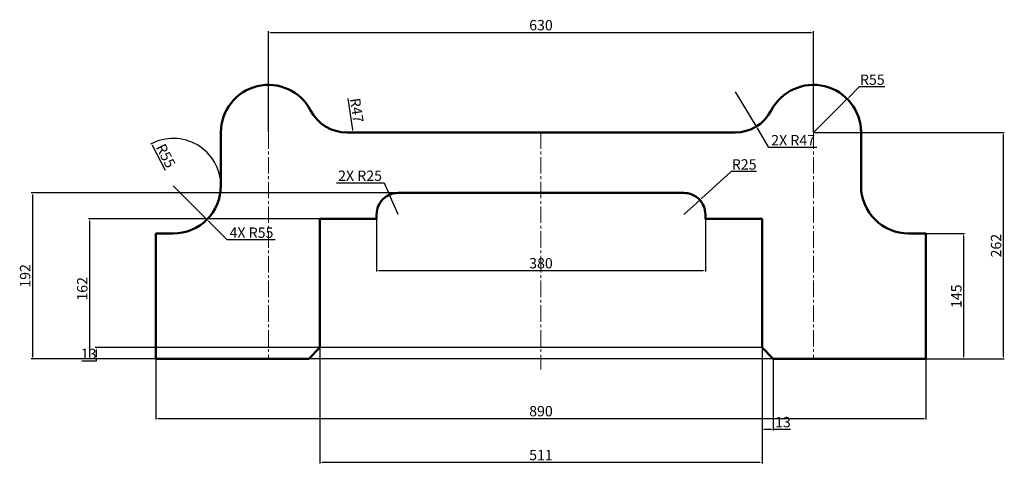
# Model space of a CAD drawing. Units: millimetres. Extents: x 47 to 1186, y 220 to 733.
import ezdxf

# ---------------------------------------------------------------- set-up
doc = ezdxf.new("R2010")
doc.units = ezdxf.units.MM
doc.linetypes.add('CENTER2', pattern=[28.575, 19.05, -3.175, 3.175, -3.175])
for name, color, linetype, lineweight in [('M-CNTR', 4, 'CENTER2', 18), ('M-DIMS', 2, 'Continuous', 25), ('M-OUTL', 7, 'Continuous', 50)]:
    doc.layers.add(name, color=color, linetype=linetype, lineweight=lineweight)
doc.styles.get("Standard").update_dxf_attribs({"font": 'arial.ttf'})
doc.dimstyles.new('ISO-25', dxfattribs={"dimtxt": 12, "dimasz": 2.5, "dimexe": 1.25, "dimexo": 0.625, "dimtad": 1, "dimtoh": 1, "dimdec": 0, "dimtxsty": 'Standard', "dimcen": 2.5, "dimadec": 0, "dimazin": 0, "dimtfac": 1, "dimtdec": 0, "dimtmove": 0, "dimatfit": 3, "dimfxl": 1, "dimarcsym": 0})

# ---------------------------------------------------------------- blocks, each defined once
blk = doc.blocks.new('*D1')
at = {"layer": 'Defpoints', "color": 0, "transparency": 16777216}
for p in [(965, 718), (335, 602.3), (965, 602.3)]:
    blk.add_point(p, dxfattribs=at)
at = {"layer": 'M-DIMS', "color": 0, "lineweight": -2, "transparency": 16777216}
for p, q in [((335, 602.9), (335, 719.3)), ((337.5, 718), (962.5, 718)), ((965, 602.9), (965, 719.3))]:
    blk.add_line(p, q, dxfattribs=at)
at = {"layer": 'M-DIMS', "color": 0, "transparency": 16777216}
for points in [[(337.5, 718.5), (337.5, 717.6), (335, 718)], [(962.5, 718.5), (962.5, 717.6), (965, 718)]]:
    blk.add_solid(points, dxfattribs=at)
at = {"layer": 'M-DIMS', "color": 0, "transparency": 16777216, "insert": (650, 724.8), "char_height": 12, "attachment_point": 5}
blk.add_mtext('630', dxfattribs=at)
blk = doc.blocks.new('*D2')
at = {"layer": 'Defpoints', "color": 0, "transparency": 16777216}
for p in [(485, 532.3), (62.1, 340.3), (205, 340.3)]:
    blk.add_point(p, dxfattribs=at)
at = {"layer": 'M-DIMS', "color": 0, "lineweight": -2, "transparency": 16777216}
for p, q in [((484.4, 532.3), (60.9, 532.3)), ((62.1, 529.8), (62.1, 342.8)), ((204.4, 340.3), (60.9, 340.3))]:
    blk.add_line(p, q, dxfattribs=at)
at = {"layer": 'M-DIMS', "color": 0, "transparency": 16777216}
for points in [[(61.7, 529.8), (62.5, 529.8), (62.1, 532.3)], [(61.7, 342.8), (62.5, 342.8), (62.1, 340.3)]]:
    blk.add_solid(points, dxfattribs=at)
at = {"layer": 'M-DIMS', "color": 0, "transparency": 16777216, "insert": (55.3, 436.3), "char_height": 12, "attachment_point": 5, "rotation": 90}
blk.add_mtext('192', dxfattribs=at)
blk = doc.blocks.new('*D3')
at = {"layer": 'Defpoints', "color": 0, "transparency": 16777216}
for p in [(460, 502.3), (128.1, 340.3), (381.5, 340.3)]:
    blk.add_point(p, dxfattribs=at)
at = {"layer": 'M-DIMS', "color": 0, "lineweight": -2, "transparency": 16777216}
for p, q in [((459.4, 502.3), (126.9, 502.3)), ((128.1, 499.8), (128.1, 342.8)), ((380.9, 340.3), (126.9, 340.3))]:
    blk.add_line(p, q, dxfattribs=at)
at = {"layer": 'M-DIMS', "color": 0, "transparency": 16777216}
for points in [[(127.7, 499.8), (128.5, 499.8), (128.1, 502.3)], [(127.7, 342.8), (128.5, 342.8), (128.1, 340.3)]]:
    blk.add_solid(points, dxfattribs=at)
at = {"layer": 'M-DIMS', "color": 0, "transparency": 16777216, "insert": (121.4, 421.3), "char_height": 12, "attachment_point": 5, "rotation": 90}
blk.add_mtext('162', dxfattribs=at)
blk = doc.blocks.new('*D4')
at = {"layer": 'Defpoints', "color": 0, "transparency": 16777216}
for p in [(199.8, 589.2), (225, 540.3)]:
    blk.add_point(p, dxfattribs=at)
at = {"layer": 'M-DIMS', "color": 0, "lineweight": -2, "transparency": 16777216}
blk.add_line((215.9, 558.1), (201, 587), dxfattribs=at)
blk.add_arc((225, 540.3), 55, 0.6511, 118.5297, dxfattribs=at)
at = {"layer": 'M-DIMS', "color": 0, "transparency": 16777216}
blk.add_solid([(201.4, 587.2), (200.6, 586.8), (199.8, 589.2)], dxfattribs=at)
at = {"layer": 'M-DIMS', "color": 0, "transparency": 16777216, "insert": (215, 574.5), "char_height": 12, "attachment_point": 5, "rotation": 297.2275}
blk.add_mtext('R55', dxfattribs=at)
blk = doc.blocks.new('*D5')
at = {"layer": 'Defpoints', "color": 0, "transparency": 16777216}
for p in [(425.5, 649.3), (432.6, 602.8)]:
    blk.add_point(p, dxfattribs=at)
at = {"layer": 'M-DIMS', "color": 0, "lineweight": -2, "transparency": 16777216}
blk.add_line((426.7, 641.4), (432.2, 605.3), dxfattribs=at)
blk.add_arc((425.5, 649.3), 47, 270.7619, 280.1996, dxfattribs=at)
at = {"layer": 'M-DIMS', "color": 0, "transparency": 16777216}
blk.add_solid([(432.7, 605.4), (431.8, 605.2), (432.6, 602.8)], dxfattribs=at)
at = {"layer": 'M-DIMS', "color": 0, "transparency": 16777216, "insert": (435.5, 627.6), "char_height": 12, "attachment_point": 5, "rotation": 278.6757}
blk.add_mtext('R47', dxfattribs=at)
blk = doc.blocks.new('*D6')
at = {"layer": 'Defpoints', "color": 0, "transparency": 16777216}
for p in [(1004, 641.1), (965, 602.3)]:
    blk.add_point(p, dxfattribs=at)
at = {"layer": 'M-DIMS', "color": 0, "lineweight": -2, "transparency": 16777216}
for p, q in [((1018, 655), (1005.8, 642.8)), ((1047.4, 655), (1018, 655)), ((965, 602.3), (1004, 641.1))]:
    blk.add_line(p, q, dxfattribs=at)
at = {"layer": 'M-DIMS', "color": 0, "transparency": 16777216}
blk.add_solid([(1005.5, 643.1), (1006.1, 642.5), (1004, 641.1)], dxfattribs=at)
at = {"layer": 'M-DIMS', "color": 0, "transparency": 16777216, "insert": (1033, 661.7), "char_height": 12, "attachment_point": 5}
blk.add_mtext('R55', dxfattribs=at)
blk = doc.blocks.new('*D7')
at = {"layer": 'Defpoints', "color": 0, "transparency": 16777216}
for p in [(833.5, 524), (815, 507.3)]:
    blk.add_point(p, dxfattribs=at)
at = {"layer": 'M-DIMS', "color": 0, "lineweight": -2, "transparency": 16777216}
for p, q in [((869.9, 556.9), (835.4, 525.7)), ((899.3, 556.9), (869.9, 556.9)), ((815, 507.3), (833.5, 524))]:
    blk.add_line(p, q, dxfattribs=at)
at = {"layer": 'M-DIMS', "color": 0, "transparency": 16777216}
blk.add_solid([(835.1, 526), (835.7, 525.4), (833.5, 524)], dxfattribs=at)
at = {"layer": 'M-DIMS', "color": 0, "transparency": 16777216, "insert": (884.9, 563.7), "char_height": 12, "attachment_point": 5}
blk.add_mtext('R25', dxfattribs=at)
blk = doc.blocks.new('*D8')
at = {"layer": 'Defpoints', "color": 0, "transparency": 16777216}
for p in [(1095, 485.3), (1095, 340.3), (1138.5, 340.3)]:
    blk.add_point(p, dxfattribs=at)
at = {"layer": 'M-DIMS', "color": 0, "lineweight": -2, "transparency": 16777216}
for p, q in [((1095.6, 485.3), (1139.7, 485.3)), ((1138.5, 482.8), (1138.5, 342.8)), ((1095.6, 340.3), (1139.7, 340.3))]:
    blk.add_line(p, q, dxfattribs=at)
at = {"layer": 'M-DIMS', "color": 0, "transparency": 16777216}
for points in [[(1138, 482.8), (1138.9, 482.8), (1138.5, 485.3)], [(1138, 342.8), (1138.9, 342.8), (1138.5, 340.3)]]:
    blk.add_solid(points, dxfattribs=at)
at = {"layer": 'M-DIMS', "color": 0, "transparency": 16777216, "insert": (1131.7, 412.8), "char_height": 12, "attachment_point": 5, "rotation": 90}
blk.add_mtext('145', dxfattribs=at)
blk = doc.blocks.new('*D9')
at = {"layer": 'Defpoints', "color": 0, "transparency": 16777216}
for p in [(965, 602.3), (965, 340.3), (1184.3, 340.3)]:
    blk.add_point(p, dxfattribs=at)
at = {"layer": 'M-DIMS', "color": 0, "lineweight": -2, "transparency": 16777216}
for p, q in [((965.6, 602.3), (1185.6, 602.3)), ((1184.3, 599.8), (1184.3, 342.8)), ((965.6, 340.3), (1185.6, 340.3))]:
    blk.add_line(p, q, dxfattribs=at)
at = {"layer": 'M-DIMS', "color": 0, "transparency": 16777216}
for points in [[(1183.9, 599.8), (1184.7, 599.8), (1184.3, 602.3)], [(1183.9, 342.8), (1184.7, 342.8), (1184.3, 340.3)]]:
    blk.add_solid(points, dxfattribs=at)
at = {"layer": 'M-DIMS', "color": 0, "transparency": 16777216, "insert": (1177.6, 471.3), "char_height": 12, "attachment_point": 5, "rotation": 90}
blk.add_mtext('262', dxfattribs=at)
blk = doc.blocks.new('*D10')
at = {"layer": 'Defpoints', "color": 0, "transparency": 16777216}
for p in [(460, 507.3), (840, 507.3), (840, 442.6)]:
    blk.add_point(p, dxfattribs=at)
at = {"layer": 'M-DIMS', "color": 0, "lineweight": -2, "transparency": 16777216}
for p, q in [((460, 506.7), (460, 441.4)), ((840, 506.7), (840, 441.4)), ((462.5, 442.6), (837.5, 442.6))]:
    blk.add_line(p, q, dxfattribs=at)
at = {"layer": 'M-DIMS', "color": 0, "transparency": 16777216}
for points in [[(462.5, 443.1), (462.5, 442.2), (460, 442.6)], [(837.5, 443.1), (837.5, 442.2), (840, 442.6)]]:
    blk.add_solid(points, dxfattribs=at)
at = {"layer": 'M-DIMS', "color": 0, "transparency": 16777216, "insert": (650, 449.4), "char_height": 12, "attachment_point": 5}
blk.add_mtext('380', dxfattribs=at)
blk = doc.blocks.new('*D11')
at = {"layer": 'Defpoints', "color": 0, "transparency": 16777216}
for p in [(394.5, 353.3), (905.5, 353.3), (905.5, 220.8)]:
    blk.add_point(p, dxfattribs=at)
at = {"layer": 'M-DIMS', "color": 0, "lineweight": -2, "transparency": 16777216}
for p, q in [((394.5, 352.7), (394.5, 219.5)), ((905.5, 352.7), (905.5, 219.5)), ((397, 220.8), (903, 220.8))]:
    blk.add_line(p, q, dxfattribs=at)
at = {"layer": 'M-DIMS', "color": 0, "transparency": 16777216}
for points in [[(397, 221.2), (397, 220.4), (394.5, 220.8)], [(903, 221.2), (903, 220.4), (905.5, 220.8)]]:
    blk.add_solid(points, dxfattribs=at)
at = {"layer": 'M-DIMS', "color": 0, "transparency": 16777216, "insert": (650, 227.5), "char_height": 12, "attachment_point": 5}
blk.add_mtext('511', dxfattribs=at)
blk = doc.blocks.new('*D12')
at = {"layer": 'Defpoints', "color": 0, "transparency": 16777216}
for p in [(205, 340.3), (1095, 340.3), (1095, 271.5)]:
    blk.add_point(p, dxfattribs=at)
at = {"layer": 'M-DIMS', "color": 0, "lineweight": -2, "transparency": 16777216}
for p, q in [((205, 339.7), (205, 270.3)), ((1095, 339.7), (1095, 270.3)), ((207.5, 271.5), (1092.5, 271.5))]:
    blk.add_line(p, q, dxfattribs=at)
at = {"layer": 'M-DIMS', "color": 0, "transparency": 16777216}
for points in [[(207.5, 271.9), (207.5, 271.1), (205, 271.5)], [(1092.5, 271.9), (1092.5, 271.1), (1095, 271.5)]]:
    blk.add_solid(points, dxfattribs=at)
at = {"layer": 'M-DIMS', "color": 0, "transparency": 16777216, "insert": (650, 278.3), "char_height": 12, "attachment_point": 5}
blk.add_mtext('890', dxfattribs=at)
blk = doc.blocks.new('*D13')
at = {"layer": 'Defpoints', "color": 0, "transparency": 16777216}
for p in [(905.5, 353.3), (135.9, 340.3), (918.5, 340.3)]:
    blk.add_point(p, dxfattribs=at)
at = {"layer": 'M-DIMS', "color": 0, "lineweight": -2, "transparency": 16777216}
for p, q in [((904.9, 353.3), (134.7, 353.3)), ((135.9, 350.8), (135.9, 342.8)), ((135.9, 337.8), (119.2, 337.8)), ((917.9, 340.3), (134.7, 340.3)), ((135.9, 340.3), (135.9, 337.8))]:
    blk.add_line(p, q, dxfattribs=at)
at = {"layer": 'M-DIMS', "color": 0, "transparency": 16777216}
for points in [[(135.5, 350.8), (136.3, 350.8), (135.9, 353.3)], [(135.5, 342.8), (136.3, 342.8), (135.9, 340.3)]]:
    blk.add_solid(points, dxfattribs=at)
at = {"layer": 'M-DIMS', "color": 0, "transparency": 16777216, "insert": (127.2, 344.5), "char_height": 12, "attachment_point": 5}
blk.add_mtext('13', dxfattribs=at)
blk = doc.blocks.new('*D14')
at = {"layer": 'Defpoints', "color": 0, "transparency": 16777216}
for p in [(905.5, 353.3), (918.5, 340.3), (918.5, 258.9)]:
    blk.add_point(p, dxfattribs=at)
at = {"layer": 'M-DIMS', "color": 0, "lineweight": -2, "transparency": 16777216}
for p, q in [((905.5, 352.7), (905.5, 257.6)), ((918.5, 339.7), (918.5, 257.6)), ((908, 258.9), (916, 258.9)), ((918.5, 258.9), (938.3, 258.9))]:
    blk.add_line(p, q, dxfattribs=at)
at = {"layer": 'M-DIMS', "color": 0, "transparency": 16777216}
for points in [[(908, 259.3), (908, 258.5), (905.5, 258.9)], [(916, 259.3), (916, 258.5), (918.5, 258.9)]]:
    blk.add_solid(points, dxfattribs=at)
at = {"layer": 'M-DIMS', "color": 0, "transparency": 16777216, "insert": (929.7, 265.6), "char_height": 12, "attachment_point": 5}
blk.add_mtext('13', dxfattribs=at)
blk = doc.blocks.new('*D15')
at = {"layer": 'Defpoints', "color": 0, "transparency": 16777216}
for p in [(225, 540.3), (263.9, 501.4)]:
    blk.add_point(p, dxfattribs=at)
at = {"layer": 'M-DIMS', "color": 0, "lineweight": -2, "transparency": 16777216}
for p, q in [((225, 540.3), (263.9, 501.4)), ((287.2, 478.1), (265.7, 499.6)), ((342.9, 478.1), (287.2, 478.1))]:
    blk.add_line(p, q, dxfattribs=at)
at = {"layer": 'M-DIMS', "color": 0, "transparency": 16777216}
blk.add_solid([(266, 499.9), (265.4, 499.3), (263.9, 501.4)], dxfattribs=at)
at = {"layer": 'M-DIMS', "color": 0, "transparency": 16777216, "insert": (315.4, 484.8), "char_height": 12, "attachment_point": 5}
blk.add_mtext('4X R55', dxfattribs=at)
blk = doc.blocks.new('*D16')
at = {"layer": 'Defpoints', "color": 0, "transparency": 16777216}
for p in [(874.5, 649.3), (898.9, 609.1)]:
    blk.add_point(p, dxfattribs=at)
at = {"layer": 'M-DIMS', "color": 0, "lineweight": -2, "transparency": 16777216}
for p, q in [((874.5, 649.3), (898.9, 609.1)), ((913.5, 585), (900.2, 607)), ((968.8, 585), (913.5, 585))]:
    blk.add_line(p, q, dxfattribs=at)
at = {"layer": 'M-DIMS', "color": 0, "transparency": 16777216}
blk.add_solid([(900.5, 607.2), (899.8, 606.8), (898.9, 609.1)], dxfattribs=at)
at = {"layer": 'M-DIMS', "color": 0, "transparency": 16777216, "insert": (941.5, 591.7), "char_height": 12, "attachment_point": 5}
blk.add_mtext('2X R47', dxfattribs=at)
blk = doc.blocks.new('*D17')
at = {"layer": 'Defpoints', "color": 0, "transparency": 16777216}
for p in [(474.9, 530.2), (485, 507.3)]:
    blk.add_point(p, dxfattribs=at)
at = {"layer": 'M-DIMS', "color": 0, "lineweight": -2, "transparency": 16777216}
for p, q in [((413.5, 543.9), (468.9, 543.9)), ((468.9, 543.9), (473.9, 532.4)), ((485, 507.3), (474.9, 530.2))]:
    blk.add_line(p, q, dxfattribs=at)
at = {"layer": 'M-DIMS', "color": 0, "transparency": 16777216}
blk.add_solid([(474.3, 532.6), (473.5, 532.3), (474.9, 530.2)], dxfattribs=at)
at = {"layer": 'M-DIMS', "color": 0, "transparency": 16777216, "insert": (440.9, 550.6), "char_height": 12, "attachment_point": 5}
blk.add_mtext('2X R25', dxfattribs=at)

msp = doc.modelspace()

# ---------------------------------------------------------------- linework, layer by layer
at = {"layer": 'M-CNTR'}
for p, q in [((335, 602.3), (335, 340.3)), ((965, 602.3), (965, 340.3))]:
    msp.add_line(p, q, dxfattribs=at)
msp.add_lwpolyline([(650, 602.3), (650, 328)], dxfattribs=at)
at = {"layer": 'M-OUTL'}
for p, q in [((225, 485.3), (225, 485.3)), ((1075, 485.3), (1075, 485.3))]:
    msp.add_line(p, q, dxfattribs=at)
msp.add_lwpolyline([(485, 532.3, 0.414214), (460, 507.3), (460, 502.3), (394.5, 502.3), (394.5, 353.3), (381.5, 340.3), (205, 340.3), (205, 485.3), (225, 485.3, 0.414214), (280, 540.3), (280, 602.3, -0.785244), (383.8, 627.6, 0.279968), (425.5, 602.3), (874.5, 602.3, 0.279968), (916.2, 627.6, -0.785244), (1020, 602.3), (1020, 540.3, 0.414214), (1075, 485.3), (1095, 485.3), (1095, 340.3), (918.5, 340.3), (905.5, 353.3), (905.5, 502.3), (840, 502.3), (840, 507.3, 0.414214), (815, 532.3)], format="xyb", close=True, dxfattribs=at)

# ---------------------------------------------------------------- dimensions: what is measured, and where the dimension line sits
at = {"layer": 'M-DIMS'}
for base, p1, p2, override, picture, middle in [((965, 718), (335, 602.3), (965, 602.3), {"dimclrd": 0, "dimclre": 0, "dimclrt": 0}, '*D1', (650, 724.8)), ((840, 442.6), (460, 507.3), (840, 507.3), {"dimclrd": 0, "dimclre": 0, "dimclrt": 0}, '*D10', (650, 449.4)), ((905.5, 220.8), (394.5, 353.3), (905.5, 353.3), {"dimclrd": 0, "dimclre": 0, "dimclrt": 0}, '*D11', (650, 227.5)), ((918.5, 258.9), (905.5, 353.3), (918.5, 340.3), {"dimdec": 0, "dimlfac": 1, "dimrnd": 0, "dimzin": 0, "dimdsep": 46, "dimlunit": 2}, '*D14', (929.7, 265.6)), ((1095, 271.5), (205, 340.3), (1095, 340.3), {"dimclrd": 0, "dimclre": 0, "dimclrt": 0}, '*D12', (650, 278.3))]:
    dim = msp.add_linear_dim(base=base, p1=p1, p2=p2, dimstyle='ISO-25', override=override, dxfattribs=at)
    dim.commit()
    dim.dimension.update_dxf_attribs({"geometry": picture, "text_midpoint": middle})
for center, mpoint, picture, middle in [((965, 602.3), (1004, 641.1), '*D6', (1033, 655)), ((425.5, 649.3), (432.6, 602.8), '*D5', (429, 626.6)), ((225, 540.3), (199.8, 589.2), '*D4', (209, 571.4)), ((815, 507.3), (833.5, 524), '*D7', (884.9, 556.9))]:
    dim = msp.add_radius_dim(center=center, mpoint=mpoint, dimstyle='ISO-25', override={"dimclrd": 0, "dimclre": 0, "dimclrt": 0}, dxfattribs=at)
    dim.commit()
    dim.dimension.update_dxf_attribs({"geometry": picture, "text_midpoint": middle, "dimtype": 164})
for center, mpoint, text, picture, middle in [((874.5, 649.3), (898.9, 609.1), '2X <>', '*D16', (941.5, 585)), ((485, 507.3), (474.9, 530.2), '2X <>', '*D17', (440.9, 543.9)), ((225, 540.3), (263.9, 501.4), '4X <>', '*D15', (315.4, 478.1))]:
    dim = msp.add_radius_dim(center=center, mpoint=mpoint, text=text, dimstyle='ISO-25', override={"dimdec": 0, "dimlfac": 1, "dimrnd": 0, "dimzin": 0, "dimdsep": 46, "dimlunit": 2}, dxfattribs=at)
    dim.commit()
    dim.dimension.update_dxf_attribs({"geometry": picture, "text_midpoint": middle, "dimtype": 164})
for base, p1, p2, override, picture, middle in [((1184.3, 340.3), (965, 602.3), (965, 340.3), {"dimclrd": 0, "dimclre": 0, "dimclrt": 0}, '*D9', (1177.6, 471.3)), ((62.1, 340.3), (485, 532.3), (205, 340.3), {"dimclrd": 0, "dimclre": 0, "dimclrt": 0}, '*D2', (55.3, 436.3)), ((128.1, 340.3), (460, 502.3), (381.5, 340.3), {"dimclrd": 0, "dimclre": 0, "dimclrt": 0}, '*D3', (121.4, 421.3)), ((1138.5, 340.3), (1095, 485.3), (1095, 340.3), {"dimclrd": 0, "dimclre": 0, "dimclrt": 0}, '*D8', (1131.7, 412.8)), ((135.9, 340.3), (905.5, 353.3), (918.5, 340.3), {"dimdec": 0, "dimlfac": 1, "dimrnd": 0, "dimzin": 0, "dimdsep": 46, "dimlunit": 2}, '*D13', (127.2, 344.5))]:
    dim = msp.add_linear_dim(base=base, p1=p1, p2=p2, angle=90, dimstyle='ISO-25', override=override, dxfattribs=at)
    dim.commit()
    dim.dimension.update_dxf_attribs({"geometry": picture, "text_midpoint": middle})

doc.saveas('drawing.dxf')
